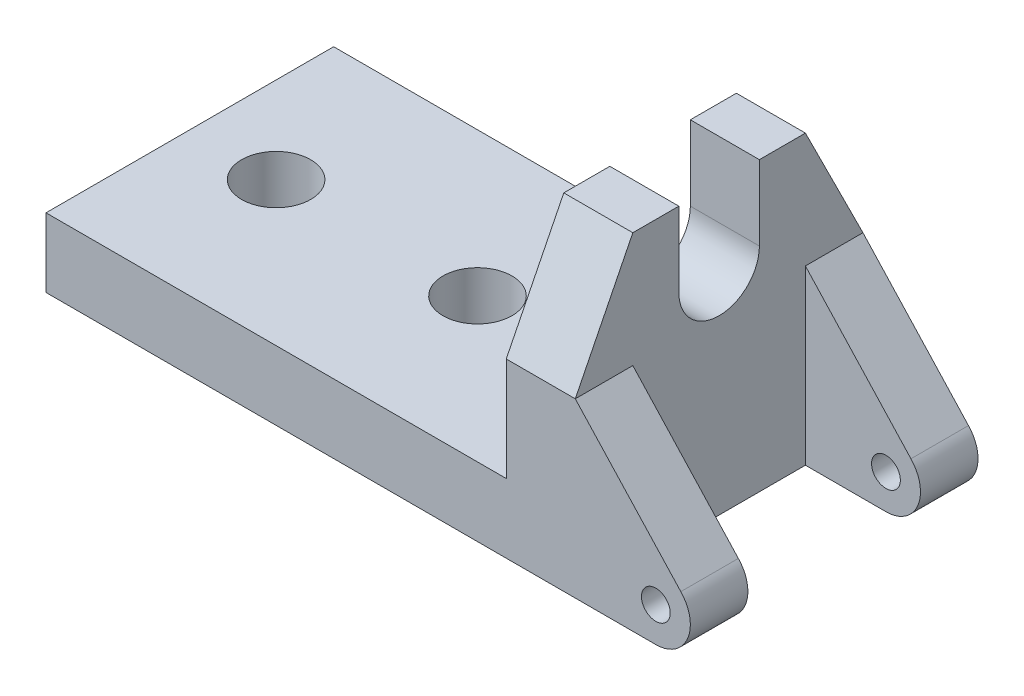
ISO-10303-21;
HEADER;
FILE_DESCRIPTION(('STEP AP214'),'2;1');
FILE_NAME('part.step','',(''),(''),'','','');
FILE_SCHEMA(('AUTOMOTIVE_DESIGN { 1 0 10303 214 1 1 1 1 }'));
ENDSEC;
DATA;
#1=APPLICATION_CONTEXT('core data for automotive mechanical design processes');
#2=APPLICATION_PROTOCOL_DEFINITION('international standard','automotive_design',2000,#1);
#3=PRODUCT_CONTEXT('',#1,'mechanical');
#4=PRODUCT('Part','Part','',(#3));
#5=PRODUCT_RELATED_PRODUCT_CATEGORY('part','',(#4));
#6=PRODUCT_DEFINITION_FORMATION('','',#4);
#7=PRODUCT_DEFINITION_CONTEXT('part definition',#1,'design');
#8=PRODUCT_DEFINITION('design','',#6,#7);
#9=PRODUCT_DEFINITION_SHAPE('','',#8);
#10=(LENGTH_UNIT() NAMED_UNIT(*) SI_UNIT(.MILLI.,.METRE.));
#11=(NAMED_UNIT(*) PLANE_ANGLE_UNIT() SI_UNIT($,.RADIAN.));
#12=(NAMED_UNIT(*) SI_UNIT($,.STERADIAN.) SOLID_ANGLE_UNIT());
#13=UNCERTAINTY_MEASURE_WITH_UNIT(LENGTH_MEASURE(1.E-05),#10,'distance_accuracy_value','');
#14=(GEOMETRIC_REPRESENTATION_CONTEXT(3) GLOBAL_UNCERTAINTY_ASSIGNED_CONTEXT((#13)) GLOBAL_UNIT_ASSIGNED_CONTEXT((#10,
#11,#12)) REPRESENTATION_CONTEXT('',''));
#15=CARTESIAN_POINT('',(0.,0.,0.));
#16=DIRECTION('',(0.,0.,1.));
#17=DIRECTION('',(1.,0.,0.));
#18=AXIS2_PLACEMENT_3D('',#15,#16,#17);
#19=CARTESIAN_POINT('',(0.,0.,25.));
#20=DIRECTION('',(1.,0.,0.));
#21=DIRECTION('',(0.,0.,-1.));
#22=AXIS2_PLACEMENT_3D('',#19,#20,#21);
#23=PLANE('',#22);
#24=DIRECTION('',(0.,-1.,0.));
#25=VECTOR('',#24,1.);
#26=CARTESIAN_POINT('',(0.,0.,0.));
#27=LINE('',#26,#25);
#28=CARTESIAN_POINT('',(0.,6.,0.));
#29=VERTEX_POINT('',#28);
#30=CARTESIAN_POINT('',(0.,0.,0.));
#31=VERTEX_POINT('',#30);
#32=EDGE_CURVE('E292',#29,#31,#27,.T.);
#33=ORIENTED_EDGE('',*,*,#32,.T.);
#34=DIRECTION('',(0.,0.,-1.));
#35=VECTOR('',#34,1.);
#36=CARTESIAN_POINT('',(0.,0.,25.));
#37=LINE('',#36,#35);
#38=CARTESIAN_POINT('',(0.,0.,25.));
#39=VERTEX_POINT('',#38);
#40=EDGE_CURVE('E11',#39,#31,#37,.T.);
#41=ORIENTED_EDGE('',*,*,#40,.F.);
#42=DIRECTION('',(0.,-1.,0.));
#43=VECTOR('',#42,1.);
#44=CARTESIAN_POINT('',(0.,0.,25.));
#45=LINE('',#44,#43);
#46=CARTESIAN_POINT('',(0.,6.,25.));
#47=VERTEX_POINT('',#46);
#48=EDGE_CURVE('E291',#47,#39,#45,.T.);
#49=ORIENTED_EDGE('',*,*,#48,.F.);
#50=DIRECTION('',(0.,0.,-1.));
#51=VECTOR('',#50,1.);
#52=CARTESIAN_POINT('',(0.,6.,25.));
#53=LINE('',#52,#51);
#54=EDGE_CURVE('E301',#47,#29,#53,.T.);
#55=ORIENTED_EDGE('',*,*,#54,.T.);
#56=EDGE_LOOP('',(#33,#41,#49,#55));
#57=FACE_BOUND('',#56,.T.);
#58=ADVANCED_FACE('F50',(#57),#23,.F.);
#59=CARTESIAN_POINT('',(0.,0.,25.));
#60=DIRECTION('',(0.,1.,0.));
#61=DIRECTION('',(0.,0.,1.));
#62=AXIS2_PLACEMENT_3D('',#59,#60,#61);
#63=PLANE('',#62);
#64=CARTESIAN_POINT('',(7.5,0.,12.5));
#65=DIRECTION('',(0.,1.,0.));
#66=DIRECTION('',(0.,0.,1.));
#67=AXIS2_PLACEMENT_3D('',#64,#65,#66);
#68=CIRCLE('',#67,3.);
#69=CARTESIAN_POINT('',(7.5,0.,15.5));
#70=VERTEX_POINT('',#69);
#71=EDGE_CURVE('E678',#70,#70,#68,.T.);
#72=ORIENTED_EDGE('',*,*,#71,.T.);
#73=EDGE_LOOP('',(#72));
#74=FACE_BOUND('',#73,.T.);
#75=CARTESIAN_POINT('',(25.,0.,12.5));
#76=DIRECTION('',(0.,1.,0.));
#77=DIRECTION('',(0.,0.,1.));
#78=AXIS2_PLACEMENT_3D('',#75,#76,#77);
#79=CIRCLE('',#78,3.);
#80=CARTESIAN_POINT('',(25.,0.,15.5));
#81=VERTEX_POINT('',#80);
#82=EDGE_CURVE('E683',#81,#81,#79,.T.);
#83=ORIENTED_EDGE('',*,*,#82,.T.);
#84=EDGE_LOOP('',(#83));
#85=FACE_BOUND('',#84,.T.);
#86=DIRECTION('',(1.,0.,0.));
#87=VECTOR('',#86,1.);
#88=CARTESIAN_POINT('',(0.,0.,0.));
#89=LINE('',#88,#87);
#90=CARTESIAN_POINT('',(53.,0.,0.));
#91=VERTEX_POINT('',#90);
#92=EDGE_CURVE('E302',#31,#91,#89,.T.);
#93=ORIENTED_EDGE('',*,*,#92,.T.);
#94=DIRECTION('',(0.,0.,-1.));
#95=VECTOR('',#94,1.);
#96=CARTESIAN_POINT('',(53.,0.,5.));
#97=LINE('',#96,#95);
#98=CARTESIAN_POINT('',(53.,0.,5.));
#99=VERTEX_POINT('',#98);
#100=EDGE_CURVE('E176',#99,#91,#97,.T.);
#101=ORIENTED_EDGE('',*,*,#100,.F.);
#102=DIRECTION('',(-1.,0.,0.));
#103=VECTOR('',#102,1.);
#104=CARTESIAN_POINT('',(46.,0.,5.));
#105=LINE('',#104,#103);
#106=CARTESIAN_POINT('',(46.,0.,5.));
#107=VERTEX_POINT('',#106);
#108=EDGE_CURVE('E183',#99,#107,#105,.T.);
#109=ORIENTED_EDGE('',*,*,#108,.T.);
#110=DIRECTION('',(0.,0.,1.));
#111=VECTOR('',#110,1.);
#112=CARTESIAN_POINT('',(46.,0.,0.));
#113=LINE('',#112,#111);
#114=CARTESIAN_POINT('',(46.,0.,20.));
#115=VERTEX_POINT('',#114);
#116=EDGE_CURVE('E68',#107,#115,#113,.T.);
#117=ORIENTED_EDGE('',*,*,#116,.T.);
#118=DIRECTION('',(1.,0.,0.));
#119=VECTOR('',#118,1.);
#120=CARTESIAN_POINT('',(46.,0.,20.));
#121=LINE('',#120,#119);
#122=CARTESIAN_POINT('',(53.,0.,20.));
#123=VERTEX_POINT('',#122);
#124=EDGE_CURVE('E210',#115,#123,#121,.T.);
#125=ORIENTED_EDGE('',*,*,#124,.T.);
#126=DIRECTION('',(0.,0.,1.));
#127=VECTOR('',#126,1.);
#128=CARTESIAN_POINT('',(53.,0.,20.));
#129=LINE('',#128,#127);
#130=CARTESIAN_POINT('',(53.,0.,25.));
#131=VERTEX_POINT('',#130);
#132=EDGE_CURVE('E219',#123,#131,#129,.T.);
#133=ORIENTED_EDGE('',*,*,#132,.T.);
#134=DIRECTION('',(1.,0.,0.));
#135=VECTOR('',#134,1.);
#136=CARTESIAN_POINT('',(0.,0.,25.));
#137=LINE('',#136,#135);
#138=EDGE_CURVE('E298',#39,#131,#137,.T.);
#139=ORIENTED_EDGE('',*,*,#138,.F.);
#140=ORIENTED_EDGE('',*,*,#40,.T.);
#141=EDGE_LOOP('',(#93,#101,#109,#117,#125,#133,#139,#140));
#142=FACE_BOUND('',#141,.T.);
#143=ADVANCED_FACE('F370',(#74,#85,#142),#63,.F.);
#144=CARTESIAN_POINT('',(0.,6.,25.));
#145=DIRECTION('',(0.,-1.,0.));
#146=DIRECTION('',(0.,0.,-1.));
#147=AXIS2_PLACEMENT_3D('',#144,#145,#146);
#148=PLANE('',#147);
#149=CARTESIAN_POINT('',(7.5,6.,12.5));
#150=DIRECTION('',(0.,1.,0.));
#151=DIRECTION('',(0.,0.,1.));
#152=AXIS2_PLACEMENT_3D('',#149,#150,#151);
#153=CIRCLE('',#152,3.);
#154=CARTESIAN_POINT('',(7.5,6.,15.5));
#155=VERTEX_POINT('',#154);
#156=EDGE_CURVE('E685',#155,#155,#153,.T.);
#157=ORIENTED_EDGE('',*,*,#156,.F.);
#158=EDGE_LOOP('',(#157));
#159=FACE_BOUND('',#158,.T.);
#160=CARTESIAN_POINT('',(25.,6.,12.5));
#161=DIRECTION('',(0.,1.,0.));
#162=DIRECTION('',(0.,0.,1.));
#163=AXIS2_PLACEMENT_3D('',#160,#161,#162);
#164=CIRCLE('',#163,3.);
#165=CARTESIAN_POINT('',(25.,6.,15.5));
#166=VERTEX_POINT('',#165);
#167=EDGE_CURVE('E676',#166,#166,#164,.T.);
#168=ORIENTED_EDGE('',*,*,#167,.F.);
#169=EDGE_LOOP('',(#168));
#170=FACE_BOUND('',#169,.T.);
#171=DIRECTION('',(-1.,0.,0.));
#172=VECTOR('',#171,1.);
#173=CARTESIAN_POINT('',(0.,6.,0.));
#174=LINE('',#173,#172);
#175=CARTESIAN_POINT('',(40.,6.,0.));
#176=VERTEX_POINT('',#175);
#177=EDGE_CURVE('E300',#176,#29,#174,.T.);
#178=ORIENTED_EDGE('',*,*,#177,.T.);
#179=ORIENTED_EDGE('',*,*,#54,.F.);
#180=DIRECTION('',(-1.,0.,0.));
#181=VECTOR('',#180,1.);
#182=CARTESIAN_POINT('',(0.,6.,25.));
#183=LINE('',#182,#181);
#184=CARTESIAN_POINT('',(40.,6.,25.));
#185=VERTEX_POINT('',#184);
#186=EDGE_CURVE('E299',#185,#47,#183,.T.);
#187=ORIENTED_EDGE('',*,*,#186,.F.);
#188=DIRECTION('',(0.,0.,-1.));
#189=VECTOR('',#188,1.);
#190=CARTESIAN_POINT('',(40.,6.,25.));
#191=LINE('',#190,#189);
#192=EDGE_CURVE('E53',#185,#176,#191,.T.);
#193=ORIENTED_EDGE('',*,*,#192,.T.);
#194=EDGE_LOOP('',(#178,#179,#187,#193));
#195=FACE_BOUND('',#194,.T.);
#196=ADVANCED_FACE('F315',(#159,#170,#195),#148,.F.);
#197=CARTESIAN_POINT('',(0.,0.,25.));
#198=DIRECTION('',(0.,0.,-1.));
#199=DIRECTION('',(-1.,0.,0.));
#200=AXIS2_PLACEMENT_3D('',#197,#198,#199);
#201=PLANE('',#200);
#202=CARTESIAN_POINT('',(53.,3.,25.));
#203=DIRECTION('',(0.,0.,1.));
#204=DIRECTION('',(1.,0.,0.));
#205=AXIS2_PLACEMENT_3D('',#202,#203,#204);
#206=CIRCLE('',#205,1.25);
#207=CARTESIAN_POINT('',(54.25,3.,25.));
#208=VERTEX_POINT('',#207);
#209=EDGE_CURVE('E198',#208,#208,#206,.T.);
#210=ORIENTED_EDGE('',*,*,#209,.F.);
#211=EDGE_LOOP('',(#210));
#212=FACE_BOUND('',#211,.T.);
#213=ORIENTED_EDGE('',*,*,#48,.T.);
#214=ORIENTED_EDGE('',*,*,#138,.T.);
#215=CARTESIAN_POINT('',(53.,3.,25.));
#216=DIRECTION('',(0.,0.,1.));
#217=DIRECTION('',(1.,0.,0.));
#218=AXIS2_PLACEMENT_3D('',#215,#216,#217);
#219=CIRCLE('',#218,3.);
#220=CARTESIAN_POINT('',(55.1710345928346,5.07041271168705,25.));
#221=VERTEX_POINT('',#220);
#222=EDGE_CURVE('E205',#131,#221,#219,.T.);
#223=ORIENTED_EDGE('',*,*,#222,.T.);
#224=DIRECTION('',(-0.678490256572755,0.734609400794624,0.));
#225=VECTOR('',#224,1.);
#226=CARTESIAN_POINT('',(46.,15.,25.));
#227=LINE('',#226,#225);
#228=CARTESIAN_POINT('',(46.,15.,25.));
#229=VERTEX_POINT('',#228);
#230=EDGE_CURVE('E206',#221,#229,#227,.T.);
#231=ORIENTED_EDGE('',*,*,#230,.T.);
#232=DIRECTION('',(-1.,0.,0.));
#233=VECTOR('',#232,1.);
#234=CARTESIAN_POINT('',(46.,15.,25.));
#235=LINE('',#234,#233);
#236=CARTESIAN_POINT('',(40.,15.,25.));
#237=VERTEX_POINT('',#236);
#238=EDGE_CURVE('E281',#229,#237,#235,.T.);
#239=ORIENTED_EDGE('',*,*,#238,.T.);
#240=DIRECTION('',(0.,-1.,0.));
#241=VECTOR('',#240,1.);
#242=CARTESIAN_POINT('',(40.,15.,25.));
#243=LINE('',#242,#241);
#244=EDGE_CURVE('E277',#237,#185,#243,.T.);
#245=ORIENTED_EDGE('',*,*,#244,.T.);
#246=ORIENTED_EDGE('',*,*,#186,.T.);
#247=EDGE_LOOP('',(#213,#214,#223,#231,#239,#245,#246));
#248=FACE_BOUND('',#247,.T.);
#249=ADVANCED_FACE('F321',(#212,#248),#201,.F.);
#250=CARTESIAN_POINT('',(0.,0.,0.));
#251=DIRECTION('',(0.,0.,-1.));
#252=DIRECTION('',(-1.,0.,0.));
#253=AXIS2_PLACEMENT_3D('',#250,#251,#252);
#254=PLANE('',#253);
#255=CARTESIAN_POINT('',(53.,3.,0.));
#256=DIRECTION('',(0.,0.,-1.));
#257=DIRECTION('',(-1.,0.,0.));
#258=AXIS2_PLACEMENT_3D('',#255,#256,#257);
#259=CIRCLE('',#258,1.25);
#260=CARTESIAN_POINT('',(51.75,3.,0.));
#261=VERTEX_POINT('',#260);
#262=EDGE_CURVE('E672',#261,#261,#259,.T.);
#263=ORIENTED_EDGE('',*,*,#262,.F.);
#264=EDGE_LOOP('',(#263));
#265=FACE_BOUND('',#264,.T.);
#266=ORIENTED_EDGE('',*,*,#32,.F.);
#267=ORIENTED_EDGE('',*,*,#177,.F.);
#268=DIRECTION('',(0.,-1.,0.));
#269=VECTOR('',#268,1.);
#270=CARTESIAN_POINT('',(40.,15.,0.));
#271=LINE('',#270,#269);
#272=CARTESIAN_POINT('',(40.,15.,0.));
#273=VERTEX_POINT('',#272);
#274=EDGE_CURVE('E284',#273,#176,#271,.T.);
#275=ORIENTED_EDGE('',*,*,#274,.F.);
#276=DIRECTION('',(-1.,0.,0.));
#277=VECTOR('',#276,1.);
#278=CARTESIAN_POINT('',(46.,15.,0.));
#279=LINE('',#278,#277);
#280=CARTESIAN_POINT('',(46.,15.,0.));
#281=VERTEX_POINT('',#280);
#282=EDGE_CURVE('E285',#281,#273,#279,.T.);
#283=ORIENTED_EDGE('',*,*,#282,.F.);
#284=DIRECTION('',(0.678490256572755,-0.734609400794624,0.));
#285=VECTOR('',#284,1.);
#286=CARTESIAN_POINT('',(46.,15.,0.));
#287=LINE('',#286,#285);
#288=CARTESIAN_POINT('',(55.1710345928346,5.07041271168705,0.));
#289=VERTEX_POINT('',#288);
#290=EDGE_CURVE('E195',#281,#289,#287,.T.);
#291=ORIENTED_EDGE('',*,*,#290,.T.);
#292=CARTESIAN_POINT('',(53.,3.,0.));
#293=DIRECTION('',(0.,0.,-1.));
#294=DIRECTION('',(-1.,0.,0.));
#295=AXIS2_PLACEMENT_3D('',#292,#293,#294);
#296=CIRCLE('',#295,3.);
#297=EDGE_CURVE('E171',#289,#91,#296,.T.);
#298=ORIENTED_EDGE('',*,*,#297,.T.);
#299=ORIENTED_EDGE('',*,*,#92,.F.);
#300=EDGE_LOOP('',(#266,#267,#275,#283,#291,#298,#299));
#301=FACE_BOUND('',#300,.T.);
#302=ADVANCED_FACE('F316',(#265,#301),#254,.T.);
#303=CARTESIAN_POINT('',(40.,15.,0.));
#304=DIRECTION('',(-1.,0.,0.));
#305=DIRECTION('',(0.,0.,1.));
#306=AXIS2_PLACEMENT_3D('',#303,#304,#305);
#307=PLANE('',#306);
#308=ORIENTED_EDGE('',*,*,#192,.F.);
#309=ORIENTED_EDGE('',*,*,#244,.F.);
#310=DIRECTION('',(0.,-0.894427190999916,0.447213595499958));
#311=VECTOR('',#310,1.);
#312=CARTESIAN_POINT('',(40.,13.,26.));
#313=LINE('',#312,#311);
#314=CARTESIAN_POINT('',(40.,25.,20.));
#315=VERTEX_POINT('',#314);
#316=EDGE_CURVE('E266',#315,#237,#313,.T.);
#317=ORIENTED_EDGE('',*,*,#316,.F.);
#318=DIRECTION('',(0.,0.,1.));
#319=VECTOR('',#318,1.);
#320=CARTESIAN_POINT('',(40.,25.,0.));
#321=LINE('',#320,#319);
#322=CARTESIAN_POINT('',(40.,25.,16.));
#323=VERTEX_POINT('',#322);
#324=EDGE_CURVE('E269',#323,#315,#321,.T.);
#325=ORIENTED_EDGE('',*,*,#324,.F.);
#326=DIRECTION('',(0.,1.,0.));
#327=VECTOR('',#326,1.);
#328=CARTESIAN_POINT('',(40.,0.,16.));
#329=LINE('',#328,#327);
#330=CARTESIAN_POINT('',(40.,18.5,16.));
#331=VERTEX_POINT('',#330);
#332=EDGE_CURVE('E259',#331,#323,#329,.T.);
#333=ORIENTED_EDGE('',*,*,#332,.F.);
#334=CARTESIAN_POINT('',(40.,18.5,12.5));
#335=DIRECTION('',(-1.,0.,0.));
#336=DIRECTION('',(0.,0.,1.));
#337=AXIS2_PLACEMENT_3D('',#334,#335,#336);
#338=CIRCLE('',#337,3.5);
#339=CARTESIAN_POINT('',(40.,18.5,9.));
#340=VERTEX_POINT('',#339);
#341=EDGE_CURVE('E245',#340,#331,#338,.T.);
#342=ORIENTED_EDGE('',*,*,#341,.F.);
#343=DIRECTION('',(0.,1.,0.));
#344=VECTOR('',#343,1.);
#345=CARTESIAN_POINT('',(40.,0.,9.));
#346=LINE('',#345,#344);
#347=CARTESIAN_POINT('',(40.,25.,9.));
#348=VERTEX_POINT('',#347);
#349=EDGE_CURVE('E234',#340,#348,#346,.T.);
#350=ORIENTED_EDGE('',*,*,#349,.T.);
#351=DIRECTION('',(0.,0.,-1.));
#352=VECTOR('',#351,1.);
#353=CARTESIAN_POINT('',(40.,25.,0.));
#354=LINE('',#353,#352);
#355=CARTESIAN_POINT('',(40.,25.,5.));
#356=VERTEX_POINT('',#355);
#357=EDGE_CURVE('E243',#348,#356,#354,.T.);
#358=ORIENTED_EDGE('',*,*,#357,.T.);
#359=DIRECTION('',(0.,-0.894427190999916,-0.447213595499958));
#360=VECTOR('',#359,1.);
#361=CARTESIAN_POINT('',(40.,3.,-6.));
#362=LINE('',#361,#360);
#363=EDGE_CURVE('E237',#356,#273,#362,.T.);
#364=ORIENTED_EDGE('',*,*,#363,.T.);
#365=ORIENTED_EDGE('',*,*,#274,.T.);
#366=EDGE_LOOP('',(#308,#309,#317,#325,#333,#342,#350,#358,#364,#365));
#367=FACE_BOUND('',#366,.T.);
#368=ADVANCED_FACE('F329',(#367),#307,.T.);
#369=CARTESIAN_POINT('',(46.,0.,0.));
#370=DIRECTION('',(1.,0.,0.));
#371=DIRECTION('',(0.,0.,-1.));
#372=AXIS2_PLACEMENT_3D('',#369,#370,#371);
#373=PLANE('',#372);
#374=DIRECTION('',(0.,0.,-1.));
#375=VECTOR('',#374,1.);
#376=CARTESIAN_POINT('',(46.,15.,5.));
#377=LINE('',#376,#375);
#378=CARTESIAN_POINT('',(46.,15.,5.));
#379=VERTEX_POINT('',#378);
#380=EDGE_CURVE('E180',#379,#281,#377,.T.);
#381=ORIENTED_EDGE('',*,*,#380,.T.);
#382=DIRECTION('',(0.,-0.894427190999916,-0.447213595499958));
#383=VECTOR('',#382,1.);
#384=CARTESIAN_POINT('',(46.,3.,-6.));
#385=LINE('',#384,#383);
#386=CARTESIAN_POINT('',(46.,25.,5.));
#387=VERTEX_POINT('',#386);
#388=EDGE_CURVE('E233',#387,#281,#385,.T.);
#389=ORIENTED_EDGE('',*,*,#388,.F.);
#390=DIRECTION('',(0.,0.,-1.));
#391=VECTOR('',#390,1.);
#392=CARTESIAN_POINT('',(46.,25.,0.));
#393=LINE('',#392,#391);
#394=CARTESIAN_POINT('',(46.,25.,9.));
#395=VERTEX_POINT('',#394);
#396=EDGE_CURVE('E238',#395,#387,#393,.T.);
#397=ORIENTED_EDGE('',*,*,#396,.F.);
#398=DIRECTION('',(0.,1.,0.));
#399=VECTOR('',#398,1.);
#400=CARTESIAN_POINT('',(46.,0.,9.));
#401=LINE('',#400,#399);
#402=CARTESIAN_POINT('',(46.,18.5,9.));
#403=VERTEX_POINT('',#402);
#404=EDGE_CURVE('E232',#403,#395,#401,.T.);
#405=ORIENTED_EDGE('',*,*,#404,.F.);
#406=CARTESIAN_POINT('',(46.,18.5,12.5));
#407=DIRECTION('',(-1.,0.,0.));
#408=DIRECTION('',(0.,0.,1.));
#409=AXIS2_PLACEMENT_3D('',#406,#407,#408);
#410=CIRCLE('',#409,3.5);
#411=CARTESIAN_POINT('',(46.,18.5,16.));
#412=VERTEX_POINT('',#411);
#413=EDGE_CURVE('E251',#403,#412,#410,.T.);
#414=ORIENTED_EDGE('',*,*,#413,.T.);
#415=DIRECTION('',(0.,1.,0.));
#416=VECTOR('',#415,1.);
#417=CARTESIAN_POINT('',(46.,0.,16.));
#418=LINE('',#417,#416);
#419=CARTESIAN_POINT('',(46.,25.,16.));
#420=VERTEX_POINT('',#419);
#421=EDGE_CURVE('E262',#412,#420,#418,.T.);
#422=ORIENTED_EDGE('',*,*,#421,.T.);
#423=DIRECTION('',(0.,0.,1.));
#424=VECTOR('',#423,1.);
#425=CARTESIAN_POINT('',(46.,25.,0.));
#426=LINE('',#425,#424);
#427=CARTESIAN_POINT('',(46.,25.,20.));
#428=VERTEX_POINT('',#427);
#429=EDGE_CURVE('E263',#420,#428,#426,.T.);
#430=ORIENTED_EDGE('',*,*,#429,.T.);
#431=DIRECTION('',(0.,-0.894427190999916,0.447213595499958));
#432=VECTOR('',#431,1.);
#433=CARTESIAN_POINT('',(46.,13.,26.));
#434=LINE('',#433,#432);
#435=EDGE_CURVE('E260',#428,#229,#434,.T.);
#436=ORIENTED_EDGE('',*,*,#435,.T.);
#437=DIRECTION('',(0.,0.,1.));
#438=VECTOR('',#437,1.);
#439=CARTESIAN_POINT('',(46.,15.,20.));
#440=LINE('',#439,#438);
#441=CARTESIAN_POINT('',(46.,15.,20.));
#442=VERTEX_POINT('',#441);
#443=EDGE_CURVE('E225',#442,#229,#440,.T.);
#444=ORIENTED_EDGE('',*,*,#443,.F.);
#445=DIRECTION('',(0.,-1.,0.));
#446=VECTOR('',#445,1.);
#447=CARTESIAN_POINT('',(46.,0.,20.));
#448=LINE('',#447,#446);
#449=EDGE_CURVE('E204',#442,#115,#448,.T.);
#450=ORIENTED_EDGE('',*,*,#449,.T.);
#451=ORIENTED_EDGE('',*,*,#116,.F.);
#452=DIRECTION('',(0.,1.,0.));
#453=VECTOR('',#452,1.);
#454=CARTESIAN_POINT('',(46.,15.,5.));
#455=LINE('',#454,#453);
#456=EDGE_CURVE('E62',#107,#379,#455,.T.);
#457=ORIENTED_EDGE('',*,*,#456,.T.);
#458=EDGE_LOOP('',(#381,#389,#397,#405,#414,#422,#430,#436,#444,#450,#451,#457));
#459=FACE_BOUND('',#458,.T.);
#460=ADVANCED_FACE('F354',(#459),#373,.T.);
#461=CARTESIAN_POINT('',(46.,18.5,12.5));
#462=DIRECTION('',(-1.,0.,0.));
#463=DIRECTION('',(0.,0.,1.));
#464=AXIS2_PLACEMENT_3D('',#461,#462,#463);
#465=CYLINDRICAL_SURFACE('',#464,3.5);
#466=ORIENTED_EDGE('',*,*,#341,.T.);
#467=DIRECTION('',(-1.,0.,0.));
#468=VECTOR('',#467,1.);
#469=CARTESIAN_POINT('',(46.,18.5,16.));
#470=LINE('',#469,#468);
#471=EDGE_CURVE('E271',#412,#331,#470,.T.);
#472=ORIENTED_EDGE('',*,*,#471,.F.);
#473=ORIENTED_EDGE('',*,*,#413,.F.);
#474=DIRECTION('',(-1.,0.,0.));
#475=VECTOR('',#474,1.);
#476=CARTESIAN_POINT('',(46.,18.5,9.));
#477=LINE('',#476,#475);
#478=EDGE_CURVE('E222',#403,#340,#477,.T.);
#479=ORIENTED_EDGE('',*,*,#478,.T.);
#480=EDGE_LOOP('',(#466,#472,#473,#479));
#481=FACE_BOUND('',#480,.T.);
#482=ADVANCED_FACE('F344',(#481),#465,.F.);
#483=CARTESIAN_POINT('',(46.,0.,16.));
#484=DIRECTION('',(0.,0.,1.));
#485=DIRECTION('',(1.,0.,0.));
#486=AXIS2_PLACEMENT_3D('',#483,#484,#485);
#487=PLANE('',#486);
#488=ORIENTED_EDGE('',*,*,#332,.T.);
#489=DIRECTION('',(-1.,0.,0.));
#490=VECTOR('',#489,1.);
#491=CARTESIAN_POINT('',(46.,25.,16.));
#492=LINE('',#491,#490);
#493=EDGE_CURVE('E280',#420,#323,#492,.T.);
#494=ORIENTED_EDGE('',*,*,#493,.F.);
#495=ORIENTED_EDGE('',*,*,#421,.F.);
#496=ORIENTED_EDGE('',*,*,#471,.T.);
#497=EDGE_LOOP('',(#488,#494,#495,#496));
#498=FACE_BOUND('',#497,.T.);
#499=ADVANCED_FACE('F336',(#498),#487,.F.);
#500=CARTESIAN_POINT('',(46.,25.,0.));
#501=DIRECTION('',(0.,-1.,0.));
#502=DIRECTION('',(0.,0.,-1.));
#503=AXIS2_PLACEMENT_3D('',#500,#501,#502);
#504=PLANE('',#503);
#505=ORIENTED_EDGE('',*,*,#324,.T.);
#506=DIRECTION('',(-1.,0.,0.));
#507=VECTOR('',#506,1.);
#508=CARTESIAN_POINT('',(46.,25.,20.));
#509=LINE('',#508,#507);
#510=EDGE_CURVE('E261',#428,#315,#509,.T.);
#511=ORIENTED_EDGE('',*,*,#510,.F.);
#512=ORIENTED_EDGE('',*,*,#429,.F.);
#513=ORIENTED_EDGE('',*,*,#493,.T.);
#514=EDGE_LOOP('',(#505,#511,#512,#513));
#515=FACE_BOUND('',#514,.T.);
#516=ADVANCED_FACE('F334',(#515),#504,.F.);
#517=CARTESIAN_POINT('',(46.,13.,26.));
#518=DIRECTION('',(0.,-0.447213595499958,-0.894427190999916));
#519=DIRECTION('',(0.,0.894427190999916,-0.447213595499958));
#520=AXIS2_PLACEMENT_3D('',#517,#518,#519);
#521=PLANE('',#520);
#522=ORIENTED_EDGE('',*,*,#316,.T.);
#523=ORIENTED_EDGE('',*,*,#238,.F.);
#524=ORIENTED_EDGE('',*,*,#435,.F.);
#525=ORIENTED_EDGE('',*,*,#510,.T.);
#526=EDGE_LOOP('',(#522,#523,#524,#525));
#527=FACE_BOUND('',#526,.T.);
#528=ADVANCED_FACE('F326',(#527),#521,.F.);
#529=CARTESIAN_POINT('',(46.,3.,-6.));
#530=DIRECTION('',(0.,0.447213595499958,-0.894427190999916));
#531=DIRECTION('',(0.,0.894427190999916,0.447213595499958));
#532=AXIS2_PLACEMENT_3D('',#529,#530,#531);
#533=PLANE('',#532);
#534=ORIENTED_EDGE('',*,*,#363,.F.);
#535=DIRECTION('',(-1.,0.,0.));
#536=VECTOR('',#535,1.);
#537=CARTESIAN_POINT('',(46.,25.,5.));
#538=LINE('',#537,#536);
#539=EDGE_CURVE('E236',#387,#356,#538,.T.);
#540=ORIENTED_EDGE('',*,*,#539,.F.);
#541=ORIENTED_EDGE('',*,*,#388,.T.);
#542=ORIENTED_EDGE('',*,*,#282,.T.);
#543=EDGE_LOOP('',(#534,#540,#541,#542));
#544=FACE_BOUND('',#543,.T.);
#545=ADVANCED_FACE('F351',(#544),#533,.T.);
#546=CARTESIAN_POINT('',(46.,25.,0.));
#547=DIRECTION('',(0.,1.,0.));
#548=DIRECTION('',(0.,0.,1.));
#549=AXIS2_PLACEMENT_3D('',#546,#547,#548);
#550=PLANE('',#549);
#551=ORIENTED_EDGE('',*,*,#357,.F.);
#552=DIRECTION('',(-1.,0.,0.));
#553=VECTOR('',#552,1.);
#554=CARTESIAN_POINT('',(46.,25.,9.));
#555=LINE('',#554,#553);
#556=EDGE_CURVE('E235',#395,#348,#555,.T.);
#557=ORIENTED_EDGE('',*,*,#556,.F.);
#558=ORIENTED_EDGE('',*,*,#396,.T.);
#559=ORIENTED_EDGE('',*,*,#539,.T.);
#560=EDGE_LOOP('',(#551,#557,#558,#559));
#561=FACE_BOUND('',#560,.T.);
#562=ADVANCED_FACE('F346',(#561),#550,.T.);
#563=CARTESIAN_POINT('',(46.,0.,9.));
#564=DIRECTION('',(0.,0.,1.));
#565=DIRECTION('',(1.,0.,0.));
#566=AXIS2_PLACEMENT_3D('',#563,#564,#565);
#567=PLANE('',#566);
#568=ORIENTED_EDGE('',*,*,#349,.F.);
#569=ORIENTED_EDGE('',*,*,#478,.F.);
#570=ORIENTED_EDGE('',*,*,#404,.T.);
#571=ORIENTED_EDGE('',*,*,#556,.T.);
#572=EDGE_LOOP('',(#568,#569,#570,#571));
#573=FACE_BOUND('',#572,.T.);
#574=ADVANCED_FACE('F348',(#573),#567,.T.);
#575=CARTESIAN_POINT('',(46.,15.,20.));
#576=DIRECTION('',(0.734609400794624,0.678490256572755,0.));
#577=DIRECTION('',(-0.678490256572755,0.734609400794624,0.));
#578=AXIS2_PLACEMENT_3D('',#575,#576,#577);
#579=PLANE('',#578);
#580=ORIENTED_EDGE('',*,*,#230,.F.);
#581=DIRECTION('',(0.,0.,1.));
#582=VECTOR('',#581,1.);
#583=CARTESIAN_POINT('',(55.1710345928346,5.07041271168705,20.));
#584=LINE('',#583,#582);
#585=CARTESIAN_POINT('',(55.1710345928346,5.07041271168705,20.));
#586=VERTEX_POINT('',#585);
#587=EDGE_CURVE('E224',#586,#221,#584,.T.);
#588=ORIENTED_EDGE('',*,*,#587,.F.);
#589=DIRECTION('',(-0.678490256572755,0.734609400794624,0.));
#590=VECTOR('',#589,1.);
#591=CARTESIAN_POINT('',(46.,15.,20.));
#592=LINE('',#591,#590);
#593=EDGE_CURVE('E211',#586,#442,#592,.T.);
#594=ORIENTED_EDGE('',*,*,#593,.T.);
#595=ORIENTED_EDGE('',*,*,#443,.T.);
#596=EDGE_LOOP('',(#580,#588,#594,#595));
#597=FACE_BOUND('',#596,.T.);
#598=ADVANCED_FACE('F407',(#597),#579,.T.);
#599=CARTESIAN_POINT('',(53.,3.,20.));
#600=DIRECTION('',(0.,0.,1.));
#601=DIRECTION('',(1.,0.,0.));
#602=AXIS2_PLACEMENT_3D('',#599,#600,#601);
#603=CYLINDRICAL_SURFACE('',#602,3.);
#604=ORIENTED_EDGE('',*,*,#222,.F.);
#605=ORIENTED_EDGE('',*,*,#132,.F.);
#606=CARTESIAN_POINT('',(53.,3.,20.));
#607=DIRECTION('',(0.,0.,1.));
#608=DIRECTION('',(1.,0.,0.));
#609=AXIS2_PLACEMENT_3D('',#606,#607,#608);
#610=CIRCLE('',#609,3.);
#611=EDGE_CURVE('E212',#123,#586,#610,.T.);
#612=ORIENTED_EDGE('',*,*,#611,.T.);
#613=ORIENTED_EDGE('',*,*,#587,.T.);
#614=EDGE_LOOP('',(#604,#605,#612,#613));
#615=FACE_BOUND('',#614,.T.);
#616=ADVANCED_FACE('F399',(#615),#603,.T.);
#617=CARTESIAN_POINT('',(53.,3.,20.));
#618=DIRECTION('',(0.,0.,1.));
#619=DIRECTION('',(1.,0.,0.));
#620=AXIS2_PLACEMENT_3D('',#617,#618,#619);
#621=PLANE('',#620);
#622=CARTESIAN_POINT('',(53.,3.,20.));
#623=DIRECTION('',(0.,0.,1.));
#624=DIRECTION('',(1.,0.,0.));
#625=AXIS2_PLACEMENT_3D('',#622,#623,#624);
#626=CIRCLE('',#625,1.25);
#627=CARTESIAN_POINT('',(54.25,3.,20.));
#628=VERTEX_POINT('',#627);
#629=EDGE_CURVE('E200',#628,#628,#626,.T.);
#630=ORIENTED_EDGE('',*,*,#629,.T.);
#631=EDGE_LOOP('',(#630));
#632=FACE_BOUND('',#631,.T.);
#633=ORIENTED_EDGE('',*,*,#449,.F.);
#634=ORIENTED_EDGE('',*,*,#593,.F.);
#635=ORIENTED_EDGE('',*,*,#611,.F.);
#636=ORIENTED_EDGE('',*,*,#124,.F.);
#637=EDGE_LOOP('',(#633,#634,#635,#636));
#638=FACE_BOUND('',#637,.T.);
#639=ADVANCED_FACE('F393',(#632,#638),#621,.F.);
#640=CARTESIAN_POINT('',(53.,3.,20.));
#641=DIRECTION('',(0.,0.,1.));
#642=DIRECTION('',(1.,0.,0.));
#643=AXIS2_PLACEMENT_3D('',#640,#641,#642);
#644=CYLINDRICAL_SURFACE('',#643,1.25);
#645=ORIENTED_EDGE('',*,*,#629,.F.);
#646=EDGE_LOOP('',(#645));
#647=FACE_BOUND('',#646,.T.);
#648=ORIENTED_EDGE('',*,*,#209,.T.);
#649=EDGE_LOOP('',(#648));
#650=FACE_BOUND('',#649,.T.);
#651=ADVANCED_FACE('F386',(#647,#650),#644,.F.);
#652=CARTESIAN_POINT('',(53.,3.,5.));
#653=DIRECTION('',(0.,0.,-1.));
#654=DIRECTION('',(-1.,0.,0.));
#655=AXIS2_PLACEMENT_3D('',#652,#653,#654);
#656=CYLINDRICAL_SURFACE('',#655,3.);
#657=ORIENTED_EDGE('',*,*,#297,.F.);
#658=DIRECTION('',(0.,0.,-1.));
#659=VECTOR('',#658,1.);
#660=CARTESIAN_POINT('',(55.1710345928346,5.07041271168705,5.));
#661=LINE('',#660,#659);
#662=CARTESIAN_POINT('',(55.1710345928346,5.07041271168705,5.));
#663=VERTEX_POINT('',#662);
#664=EDGE_CURVE('E165',#663,#289,#661,.T.);
#665=ORIENTED_EDGE('',*,*,#664,.F.);
#666=CARTESIAN_POINT('',(53.,3.,5.));
#667=DIRECTION('',(0.,0.,-1.));
#668=DIRECTION('',(-1.,0.,0.));
#669=AXIS2_PLACEMENT_3D('',#666,#667,#668);
#670=CIRCLE('',#669,3.);
#671=EDGE_CURVE('E166',#663,#99,#670,.T.);
#672=ORIENTED_EDGE('',*,*,#671,.T.);
#673=ORIENTED_EDGE('',*,*,#100,.T.);
#674=EDGE_LOOP('',(#657,#665,#672,#673));
#675=FACE_BOUND('',#674,.T.);
#676=ADVANCED_FACE('F168',(#675),#656,.T.);
#677=CARTESIAN_POINT('',(46.,15.,5.));
#678=DIRECTION('',(0.734609400794624,0.678490256572755,0.));
#679=DIRECTION('',(-0.678490256572755,0.734609400794624,0.));
#680=AXIS2_PLACEMENT_3D('',#677,#678,#679);
#681=PLANE('',#680);
#682=ORIENTED_EDGE('',*,*,#290,.F.);
#683=ORIENTED_EDGE('',*,*,#380,.F.);
#684=DIRECTION('',(0.678490256572755,-0.734609400794624,0.));
#685=VECTOR('',#684,1.);
#686=CARTESIAN_POINT('',(46.,15.,5.));
#687=LINE('',#686,#685);
#688=EDGE_CURVE('E185',#379,#663,#687,.T.);
#689=ORIENTED_EDGE('',*,*,#688,.T.);
#690=ORIENTED_EDGE('',*,*,#664,.T.);
#691=EDGE_LOOP('',(#682,#683,#689,#690));
#692=FACE_BOUND('',#691,.T.);
#693=ADVANCED_FACE('F187',(#692),#681,.T.);
#694=CARTESIAN_POINT('',(53.,3.,5.));
#695=DIRECTION('',(0.,0.,-1.));
#696=DIRECTION('',(-1.,0.,0.));
#697=AXIS2_PLACEMENT_3D('',#694,#695,#696);
#698=PLANE('',#697);
#699=CARTESIAN_POINT('',(53.,3.,5.));
#700=DIRECTION('',(0.,0.,-1.));
#701=DIRECTION('',(-1.,0.,0.));
#702=AXIS2_PLACEMENT_3D('',#699,#700,#701);
#703=CIRCLE('',#702,1.25);
#704=CARTESIAN_POINT('',(51.75,3.,5.));
#705=VERTEX_POINT('',#704);
#706=EDGE_CURVE('E191',#705,#705,#703,.T.);
#707=ORIENTED_EDGE('',*,*,#706,.T.);
#708=EDGE_LOOP('',(#707));
#709=FACE_BOUND('',#708,.T.);
#710=ORIENTED_EDGE('',*,*,#456,.F.);
#711=ORIENTED_EDGE('',*,*,#108,.F.);
#712=ORIENTED_EDGE('',*,*,#671,.F.);
#713=ORIENTED_EDGE('',*,*,#688,.F.);
#714=EDGE_LOOP('',(#710,#711,#712,#713));
#715=FACE_BOUND('',#714,.T.);
#716=ADVANCED_FACE('F181',(#709,#715),#698,.F.);
#717=CARTESIAN_POINT('',(53.,3.,5.));
#718=DIRECTION('',(0.,0.,-1.));
#719=DIRECTION('',(-1.,0.,0.));
#720=AXIS2_PLACEMENT_3D('',#717,#718,#719);
#721=CYLINDRICAL_SURFACE('',#720,1.25);
#722=ORIENTED_EDGE('',*,*,#706,.F.);
#723=EDGE_LOOP('',(#722));
#724=FACE_BOUND('',#723,.T.);
#725=ORIENTED_EDGE('',*,*,#262,.T.);
#726=EDGE_LOOP('',(#725));
#727=FACE_BOUND('',#726,.T.);
#728=ADVANCED_FACE('F450',(#724,#727),#721,.F.);
#729=CARTESIAN_POINT('',(25.,0.,12.5));
#730=DIRECTION('',(0.,1.,0.));
#731=DIRECTION('',(0.,0.,1.));
#732=AXIS2_PLACEMENT_3D('',#729,#730,#731);
#733=CYLINDRICAL_SURFACE('',#732,3.);
#734=ORIENTED_EDGE('',*,*,#82,.F.);
#735=EDGE_LOOP('',(#734));
#736=FACE_BOUND('',#735,.T.);
#737=ORIENTED_EDGE('',*,*,#167,.T.);
#738=EDGE_LOOP('',(#737));
#739=FACE_BOUND('',#738,.T.);
#740=ADVANCED_FACE('F452',(#736,#739),#733,.F.);
#741=CARTESIAN_POINT('',(7.5,0.,12.5));
#742=DIRECTION('',(0.,1.,0.));
#743=DIRECTION('',(0.,0.,1.));
#744=AXIS2_PLACEMENT_3D('',#741,#742,#743);
#745=CYLINDRICAL_SURFACE('',#744,3.);
#746=ORIENTED_EDGE('',*,*,#71,.F.);
#747=EDGE_LOOP('',(#746));
#748=FACE_BOUND('',#747,.T.);
#749=ORIENTED_EDGE('',*,*,#156,.T.);
#750=EDGE_LOOP('',(#749));
#751=FACE_BOUND('',#750,.T.);
#752=ADVANCED_FACE('F461',(#748,#751),#745,.F.);
#753=CLOSED_SHELL('',(#58,#143,#196,#249,#302,#368,#460,#482,#499,#516,#528,#545,#562,#574,#598,
#616,#639,#651,#676,#693,#716,#728,#740,#752));
#754=MANIFOLD_SOLID_BREP('B2',#753);
#755=ADVANCED_BREP_SHAPE_REPRESENTATION('',(#18,#754),#14);
#756=SHAPE_DEFINITION_REPRESENTATION(#9,#755);
ENDSEC;
END-ISO-10303-21;
